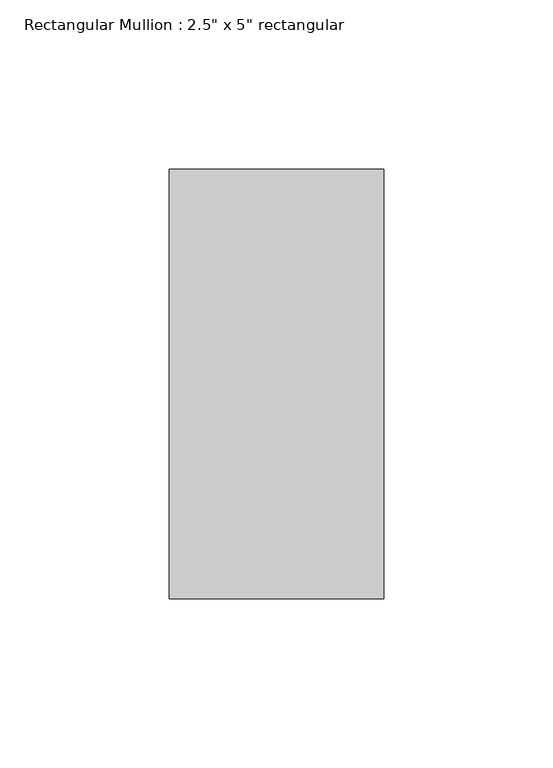
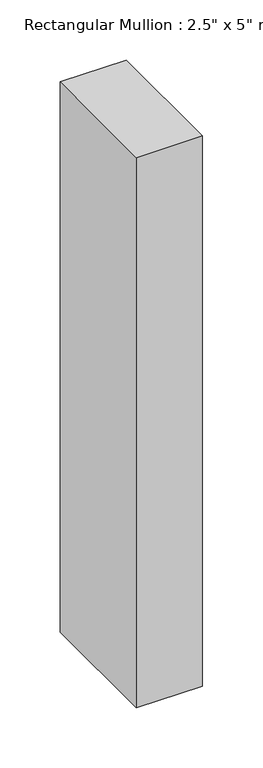
"""IFC4 building model written with IfcOpenShell, lengths in millimetres: member geometry."""

from ifc_helpers import new_model, si_unit, frame, origin, place, context, project, spatial, polyline, outline, extrude, source, transform, mapped, element, save


def member_50cacee6(model_context):
    return source(origin(), model_context, "Body", "SweptSolid", [
        extrude(outline(polyline([(0.0, 63.5), (0.0, -63.5), (-63.5, -63.5), (-63.5, 63.5), (0.0, 63.5)])), frame((0.0, 0.0, -558.8), z_axis=(0.0, 0.0, 1.0), x_axis=(1.0, 0.0, 0.0)), (0.0, 0.0, 1.0), 558.8),
    ])


if __name__ == "__main__":
    model = new_model("IFC4")
    model_context = context("Model", 3, world=origin())
    ifc_project = project(units=[si_unit("LENGTHUNIT", "METRE", prefix="MILLI")], contexts=[model_context])
    site = spatial("IfcSite", under=ifc_project)
    building = spatial("IfcBuilding", under=site)
    placement = place(None, origin())
    member_shape = member_50cacee6(model_context)
    element("IfcMember", 1, ObjectType="Rectangular Mullion : 2.5\" x 5\" rectangular", at=placement, inside=building, context=model_context, shape_type="MappedRepresentation", body=[
        mapped(member_shape, transform((0.0, 0.0, 0.0), x_axis=(1.0, 0.0, 0.0), y_axis=(0.0, 1.0, 0.0), z_axis=(0.0, 0.0, 1.0))),
    ])
    save(model, "model.ifc")

# Revit data of these elements
# Type "Rectangular Mullion : 2.5\" x 5\" rectangular"
#   built-in parameter 1007304 = 0.416667 (stored number, unit not read)
#   built-in parameter 1007301 = 0.104167 (stored number, unit not read)
#   built-in parameter 1007300 = 0.104167 (stored number, unit not read)
# Element 1 (IfcMember, "Rectangular Mullion : 2.5\" x 5\" rectangular")
#   Materials on its faces: "Aluminum"
# Materials
#   "Aluminum": class "Metal", colour RGB 247 247 247, transparency 0, Description = "Aluminum 6061", Cost = 0
